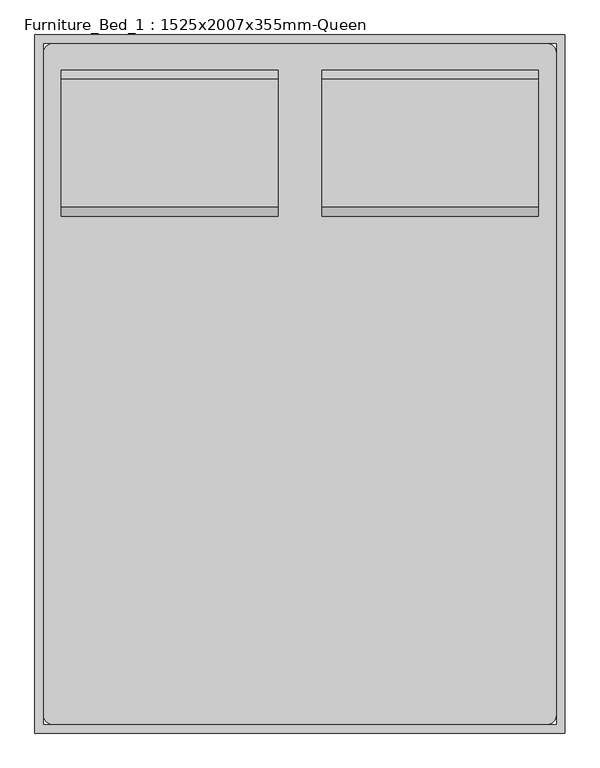
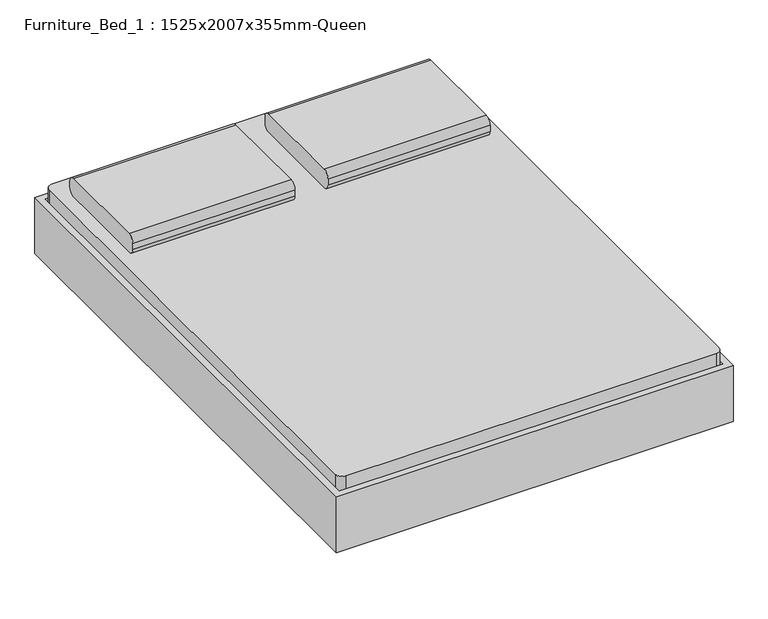
"""IFC4 building model written with IfcOpenShell, lengths in millimetres: furniture geometry, Furniture_Bed_1 : 1525x2007x355mm-Queen."""

from ifc_helpers import new_model, si_unit, point, frame, frame_2d, origin, place, context, project, spatial, polyline, circle_curve, trimmed, segment, composite_curve, outline, extrude, source, transform, mapped, element, save
from ifc_brep_helpers import plane_surface, cylinder_surface, revolved_surface, advanced_brep


def furniture_bed_1_1525x2007x355mm_queen_b7403446(model_context):
    return source(origin(), model_context, "Body", "SolidModel", [
        advanced_brep(
        [(-397.947541, -933.1295082, 196.85), (-397.947541, -933.1295082, 177.8), (-397.947541, -1009.3295082, 177.8), (-397.947541, -1009.3295082, 196.85), (-335.0113525, -933.1295082, 196.85), (-347.147541, -933.1295082, 177.8), (-347.147541, -1009.3295082, 177.8), (-335.0113525, -1009.3295082, 196.85), (-253.8115092, -933.1295082, 22.716374), (-271.0766725, -933.1295082, 14.6654962), (-271.0766725, -1009.3295082, 14.6654962), (-253.8115092, -1009.3295082, 22.716374), (-248.0564547, -933.1295082, 0.0), (-248.0564547, -933.1295082, 19.05), (-248.0564547, -1009.3295082, 0.0), (-248.0564547, -1009.3295082, 19.05), (-169.4439489, -933.1295082, 19.05), (-169.4439489, -933.1295082, 0.0), (-169.4439489, -1009.3295082, 0.0), (-169.4439489, -1009.3295082, 19.05), (-156.7439489, -933.1295082, 3.4029547), (-166.2689489, -933.1295082, 19.9007387), (-156.7439489, -1009.3295082, 3.4029547), (-166.2689489, -1009.3295082, 19.9007387), (-101.7513357, -933.1295082, 57.15), (-96.6469036, -933.1295082, 38.1), (-96.6469036, -1009.3295082, 38.1), (-101.7513357, -1009.3295082, 57.15), (780.0562537, -933.1295082, 57.15), (774.9518216, -933.1295082, 38.1), (774.9518216, -1009.3295082, 38.1), (780.0562537, -1009.3295082, 57.15), (844.5738669, -933.1295082, 19.9007387), (835.0488669, -933.1295082, 3.4029547), (835.0488669, -1009.3295082, 3.4029547), (844.5738669, -1009.3295082, 19.9007387), (847.7488669, -933.1295082, 0.0), (847.7488669, -933.1295082, 19.05), (847.7488669, -1009.3295082, 0.0), (847.7488669, -1009.3295082, 19.05), (926.3613728, -933.1295082, 19.05), (926.3613728, -933.1295082, 0.0), (926.3613728, -1009.3295082, 0.0), (926.3613728, -1009.3295082, 19.05), (949.3815906, -933.1295082, 14.6654962), (932.1164272, -933.1295082, 22.716374), (949.3815906, -1009.3295082, 14.6654962), (932.1164272, -1009.3295082, 22.716374), (1013.3162705, -933.1295082, 196.85), (1025.452459, -933.1295082, 177.8), (1025.452459, -1009.3295082, 177.8), (1013.3162705, -1009.3295082, 196.85), (1076.252459, -933.1295082, 196.85), (1076.252459, -1009.3295082, 196.85), (1076.252459, -1009.3295082, 177.8), (1076.252459, -933.1295082, 177.8)],
        [
            (0, 1),
            (1, 2),
            (2, 3),
            (3, 0),
            (0, 4),
            (4, 5),
            (5, 1),
            (5, 6),
            (6, 2),
            (6, 7),
            (7, 3),
            (7, 4),
            (4, 8),
            (8, 9),
            (9, 5),
            (9, 10),
            (10, 6),
            (10, 11),
            (11, 7),
            (11, 8),
            (12, 9, circle_curve(frame((-248.0564547, -933.1295082, 25.4), z_axis=(0.0, 1.0, 0.0), x_axis=(-0.9063077870366627, 0.0, -0.42261826174067213)), 25.4)),
            (8, 13, circle_curve(frame((-248.0564547, -933.1295082, 25.4), z_axis=(0.0, -1.0, 0.0), x_axis=(-0.9063077870366627, 0.0, -0.42261826174067213)), 6.35)),
            (13, 12),
            (14, 10, circle_curve(frame((-248.0564547, -1009.3295082, 25.4), z_axis=(0.0, 1.0, 0.0), x_axis=(-0.9063077870366627, 0.0, -0.42261826174067213)), 25.4)),
            (12, 14),
            (15, 11, circle_curve(frame((-248.0564547, -1009.3295082, 25.4), z_axis=(0.0, 1.0, 0.0), x_axis=(-0.9063077870366627, 0.0, -0.42261826174067213)), 6.35)),
            (14, 15),
            (15, 13),
            (13, 16),
            (16, 17),
            (17, 12),
            (17, 18),
            (18, 14),
            (18, 19),
            (19, 15),
            (19, 16),
            (20, 17, circle_curve(frame((-169.4439489, -933.1295082, 25.4), z_axis=(0.0, 1.0, 0.0), x_axis=(0.0, 0.0, -1.0)), 25.4)),
            (16, 21, circle_curve(frame((-169.4439489, -933.1295082, 25.4), z_axis=(0.0, -1.0, 0.0), x_axis=(0.0, 0.0, -1.0)), 6.35)),
            (21, 20),
            (22, 18, circle_curve(frame((-169.4439489, -1009.3295082, 25.4), z_axis=(0.0, 1.0, 0.0), x_axis=(0.0, 0.0, -1.0)), 25.4)),
            (20, 22),
            (23, 19, circle_curve(frame((-169.4439489, -1009.3295082, 25.4), z_axis=(0.0, 1.0, 0.0), x_axis=(0.0, 0.0, -1.0)), 6.35)),
            (22, 23),
            (23, 21),
            (21, 24),
            (24, 25),
            (25, 20),
            (25, 26),
            (26, 22),
            (26, 27),
            (27, 23),
            (27, 24),
            (24, 28),
            (28, 29),
            (29, 25),
            (29, 30),
            (30, 26),
            (30, 31),
            (31, 27),
            (31, 28),
            (28, 32),
            (32, 33),
            (33, 29),
            (33, 34),
            (34, 30),
            (34, 35),
            (35, 31),
            (35, 32),
            (36, 33, circle_curve(frame((847.7488669, -933.1295082, 25.4), z_axis=(0.0, 1.0, 0.0), x_axis=(-0.5000000000000486, 0.0, -0.8660254037844105)), 25.4)),
            (32, 37, circle_curve(frame((847.7488669, -933.1295082, 25.4), z_axis=(0.0, -1.0, 0.0), x_axis=(-0.5000000000000486, 0.0, -0.8660254037844105)), 6.35)),
            (37, 36),
            (38, 34, circle_curve(frame((847.7488669, -1009.3295082, 25.4), z_axis=(0.0, 1.0, 0.0), x_axis=(-0.5000000000000486, 0.0, -0.8660254037844105)), 25.4)),
            (36, 38),
            (39, 35, circle_curve(frame((847.7488669, -1009.3295082, 25.4), z_axis=(0.0, 1.0, 0.0), x_axis=(-0.5000000000000486, 0.0, -0.8660254037844105)), 6.35)),
            (38, 39),
            (39, 37),
            (37, 40),
            (40, 41),
            (41, 36),
            (41, 42),
            (42, 38),
            (42, 43),
            (43, 39),
            (43, 40),
            (44, 41, circle_curve(frame((926.3613728, -933.1295082, 25.4), z_axis=(0.0, 1.0, 0.0), x_axis=(0.0, 0.0, -1.0)), 25.4)),
            (40, 45, circle_curve(frame((926.3613728, -933.1295082, 25.4), z_axis=(0.0, -1.0, 0.0), x_axis=(0.0, 0.0, -1.0)), 6.35)),
            (45, 44),
            (46, 42, circle_curve(frame((926.3613728, -1009.3295082, 25.4), z_axis=(0.0, 1.0, 0.0), x_axis=(0.0, 0.0, -1.0)), 25.4)),
            (44, 46),
            (47, 43, circle_curve(frame((926.3613728, -1009.3295082, 25.4), z_axis=(0.0, 1.0, 0.0), x_axis=(0.0, 0.0, -1.0)), 6.35)),
            (46, 47),
            (47, 45),
            (45, 48),
            (48, 49),
            (49, 44),
            (49, 50),
            (50, 46),
            (50, 51),
            (51, 47),
            (51, 48),
            (52, 53),
            (53, 54),
            (54, 55),
            (55, 52),
            (48, 52),
            (55, 49),
            (54, 50),
            (53, 51),
        ],
        [
            plane_surface(frame((-397.947541, -1237.9295082, -127.5947323), z_axis=(-1.0, 0.0, 0.0), x_axis=(0.0, 1.0, 0.0))),
            plane_surface(frame((-397.947541, -933.1295082, 196.85), z_axis=(0.0, 1.0, 0.0), x_axis=(1.0, 0.0, 0.0))),
            plane_surface(frame((-397.947541, -933.1295082, 177.8), z_axis=(0.0, 0.0, -1.0), x_axis=(1.0, 0.0, 0.0))),
            plane_surface(frame((-397.947541, -1009.3295082, 177.8), z_axis=(0.0, -1.0, 0.0), x_axis=(1.0, 0.0, 0.0))),
            plane_surface(frame((-397.947541, -1009.3295082, 196.85), z_axis=(0.0, 0.0, 1.0), x_axis=(1.0, 0.0, 0.0))),
            plane_surface(frame((-335.0113525, -933.1295082, 196.85), z_axis=(0.0, 1.0000000000000002, 0.0), x_axis=(0.4226182617406718, 0.0, -0.9063077870366629))),
            plane_surface(frame((-347.147541, -933.1295082, 177.8), z_axis=(-0.906307787036663, 0.0, -0.4226182617406716), x_axis=(0.4226182617406716, 0.0, -0.906307787036663))),
            plane_surface(frame((-347.147541, -1009.3295082, 177.8), z_axis=(0.0, -1.0000000000000002, 0.0), x_axis=(0.4226182617406718, 0.0, -0.9063077870366629))),
            plane_surface(frame((-335.0113525, -1009.3295082, 196.85), z_axis=(0.9063077870366628, 0.0, 0.42261826174067196), x_axis=(0.42261826174067196, 0.0, -0.9063077870366628))),
            plane_surface(frame((-248.0564547, -933.1295082, 25.4), z_axis=(0.0, 1.0, 0.0), x_axis=(-0.9063077870366627, 0.0, -0.42261826174067213))),
            cylinder_surface(frame((-248.0564547, -1237.9295082, 25.4), z_axis=(0.0, -1.0, 0.0), x_axis=(-0.9063077870366627, 0.0, -0.42261826174067213)), 25.4),
            plane_surface(frame((-248.0564547, -1009.3295082, 25.4), z_axis=(0.0, -1.0, 0.0), x_axis=(-0.9063077870366627, 0.0, -0.42261826174067213))),
            revolved_surface(polyline([(-253.81150914768278, -1009.3295082, 22.716374037946732), (-253.81150914768278, -933.1295082, 22.716374037946732)]), (-248.0564547, -1237.9295082, 25.4), (0.0, -1.0, 0.0)),
            plane_surface(frame((-248.0564547, -933.1295082, 19.05), z_axis=(0.0, 1.0, 0.0), x_axis=(1.0, 0.0, 0.0))),
            plane_surface(frame((-248.0564547, -933.1295082, 0.0), z_axis=(0.0, 0.0, -1.0), x_axis=(1.0, 0.0, 0.0))),
            plane_surface(frame((-248.0564547, -1009.3295082, 0.0), z_axis=(0.0, -1.0, 0.0), x_axis=(1.0, 0.0, 0.0))),
            plane_surface(frame((-248.0564547, -1009.3295082, 19.05), z_axis=(0.0, 0.0, 1.0), x_axis=(1.0, 0.0, 0.0))),
            plane_surface(frame((-169.4439489, -933.1295082, 25.4), z_axis=(0.0, 1.0, 0.0), x_axis=(0.0, 0.0, -1.0))),
            cylinder_surface(frame((-169.4439489, -1237.9295082, 25.4), z_axis=(0.0, -1.0, 0.0), x_axis=(0.0, 0.0, -1.0)), 25.4),
            plane_surface(frame((-169.4439489, -1009.3295082, 25.4), z_axis=(0.0, -1.0, 0.0), x_axis=(0.0, 0.0, -1.0))),
            revolved_surface(polyline([(-169.4439489, -1009.3295082, 19.049999999999997), (-169.4439489, -933.1295082, 19.049999999999997)]), (-169.4439489, -1237.9295082, 25.4), (0.0, -1.0, 0.0)),
            plane_surface(frame((-166.2689489, -933.1295082, 19.9007387), z_axis=(0.0, 1.0, 0.0), x_axis=(0.8660254037844786, 0.0, 0.4999999999999309))),
            plane_surface(frame((-156.7439489, -933.1295082, 3.4029547), z_axis=(0.4999999999999315, 0.0, -0.8660254037844782), x_axis=(0.8660254037844782, 0.0, 0.4999999999999315))),
            plane_surface(frame((-156.7439489, -1009.3295082, 3.4029547), z_axis=(0.0, -1.0, 0.0), x_axis=(0.8660254037844788, 0.0, 0.49999999999993044))),
            plane_surface(frame((-166.2689489, -1009.3295082, 19.9007387), z_axis=(-0.4999999999999304, 0.0, 0.8660254037844789), x_axis=(0.8660254037844789, 0.0, 0.4999999999999304))),
            plane_surface(frame((-101.7513357, -933.1295082, 57.15), z_axis=(0.0, 1.0, 0.0), x_axis=(1.0, 0.0, 0.0))),
            plane_surface(frame((-96.6469036, -933.1295082, 38.1), z_axis=(0.0, 0.0, -1.0), x_axis=(1.0, 0.0, 0.0))),
            plane_surface(frame((-96.6469036, -1009.3295082, 38.1), z_axis=(0.0, -1.0, 0.0), x_axis=(1.0, 0.0, 0.0))),
            plane_surface(frame((-101.7513357, -1009.3295082, 57.15), z_axis=(0.0, 0.0, 1.0), x_axis=(1.0, 0.0, 0.0))),
            plane_surface(frame((780.0562537, -933.1295082, 57.15), z_axis=(0.0, 1.0, 0.0), x_axis=(0.866025403784412, 0.0, -0.5000000000000463))),
            plane_surface(frame((774.9518216, -933.1295082, 38.1), z_axis=(-0.500000000000047, 0.0, -0.8660254037844116), x_axis=(0.8660254037844116, 0.0, -0.500000000000047))),
            plane_surface(frame((774.9518216, -1009.3295082, 38.1), z_axis=(0.0, -1.0, 0.0), x_axis=(0.866025403784411, 0.0, -0.5000000000000481))),
            plane_surface(frame((780.0562537, -1009.3295082, 57.15), z_axis=(0.5000000000000471, 0.0, 0.8660254037844115), x_axis=(0.8660254037844115, 0.0, -0.5000000000000471))),
            plane_surface(frame((847.7488669, -933.1295082, 25.4), z_axis=(0.0, 1.0000000000000002, 0.0), x_axis=(-0.5000000000000487, 0.0, -0.8660254037844106))),
            cylinder_surface(frame((847.7488669, -1237.9295082, 25.4), z_axis=(0.0, -1.0, 0.0), x_axis=(-0.5000000000000486, 0.0, -0.8660254037844105)), 25.4),
            plane_surface(frame((847.7488669, -1009.3295082, 25.4), z_axis=(0.0, -1.0000000000000002, 0.0), x_axis=(-0.5000000000000487, 0.0, -0.8660254037844106))),
            revolved_surface(polyline([(844.5738668999998, -1009.3295082, 19.900738685968992), (844.5738668999998, -933.1295082, 19.900738685968992)]), (847.7488669, -1237.9295082, 25.4), (0.0, -1.0, 0.0)),
            plane_surface(frame((847.7488669, -933.1295082, 19.05), z_axis=(0.0, 1.0, 0.0), x_axis=(1.0, 0.0, 0.0))),
            plane_surface(frame((847.7488669, -933.1295082, 0.0), z_axis=(0.0, 0.0, -1.0), x_axis=(1.0, 0.0, 0.0))),
            plane_surface(frame((847.7488669, -1009.3295082, 0.0), z_axis=(0.0, -1.0, 0.0), x_axis=(1.0, 0.0, 0.0))),
            plane_surface(frame((847.7488669, -1009.3295082, 19.05), z_axis=(0.0, 0.0, 1.0), x_axis=(1.0, 0.0, 0.0))),
            plane_surface(frame((926.3613728, -933.1295082, 25.4), z_axis=(0.0, 1.0, 0.0), x_axis=(0.0, 0.0, -1.0))),
            cylinder_surface(frame((926.3613728, -1237.9295082, 25.4), z_axis=(0.0, -1.0, 0.0), x_axis=(0.0, 0.0, -1.0)), 25.4),
            plane_surface(frame((926.3613728, -1009.3295082, 25.4), z_axis=(0.0, -1.0, 0.0), x_axis=(0.0, 0.0, -1.0))),
            revolved_surface(polyline([(926.3613728, -1009.3295082, 19.049999999999997), (926.3613728, -933.1295082, 19.049999999999997)]), (926.3613728, -1237.9295082, 25.4), (0.0, -1.0, 0.0)),
            plane_surface(frame((932.1164272, -933.1295082, 22.716374), z_axis=(0.0, 1.0, 0.0), x_axis=(0.4226182617405395, 0.0, 0.9063077870367245))),
            plane_surface(frame((949.3815906, -933.1295082, 14.6654962), z_axis=(0.9063077870367247, 0.0, -0.4226182617405394), x_axis=(0.4226182617405394, 0.0, 0.9063077870367247))),
            plane_surface(frame((949.3815906, -1009.3295082, 14.6654962), z_axis=(0.0, -1.0, 0.0), x_axis=(0.4226182617405393, 0.0, 0.9063077870367247))),
            plane_surface(frame((932.1164272, -1009.3295082, 22.716374), z_axis=(-0.9063077870367245, 0.0, 0.42261826174053974), x_axis=(0.42261826174053974, 0.0, 0.9063077870367245))),
            plane_surface(frame((1076.252459, -1237.9295082, -127.5947323), z_axis=(1.0, 0.0, 0.0), x_axis=(0.0, 1.0, 0.0))),
            plane_surface(frame((1013.3162705, -933.1295082, 196.85), z_axis=(0.0, 1.0, 0.0), x_axis=(1.0, 0.0, 0.0))),
            plane_surface(frame((1025.452459, -933.1295082, 177.8), z_axis=(0.0, 0.0, -1.0), x_axis=(1.0, 0.0, 0.0))),
            plane_surface(frame((1025.452459, -1009.3295082, 177.8), z_axis=(0.0, -1.0, 0.0), x_axis=(1.0, 0.0, 0.0))),
            plane_surface(frame((1013.3162705, -1009.3295082, 196.85), z_axis=(0.0, 0.0, 1.0), x_axis=(1.0, 0.0, 0.0))),
        ],
        [
            (0, [[1, 2, 3, 4]]),
            (1, [[-1, 5, 6, 7]]),
            (2, [[-2, -7, 8, 9]]),
            (3, [[-3, -9, 10, 11]]),
            (4, [[-4, -11, 12, -5]]),
            (5, [[-6, 13, 14, 15]]),
            (6, [[-8, -15, 16, 17]]),
            (7, [[-10, -17, 18, 19]]),
            (8, [[-12, -19, 20, -13]]),
            (9, [[21, -14, 22, 23]]),
            (10, [[24, -16, -21, 25]]),
            (11, [[26, -18, -24, 27]]),
            (12, [[-22, -20, -26, 28]]),
            (13, [[-23, 29, 30, 31]]),
            (14, [[-25, -31, 32, 33]]),
            (15, [[-27, -33, 34, 35]]),
            (16, [[-28, -35, 36, -29]]),
            (17, [[37, -30, 38, 39]]),
            (18, [[40, -32, -37, 41]]),
            (19, [[42, -34, -40, 43]]),
            (20, [[-38, -36, -42, 44]]),
            (21, [[-39, 45, 46, 47]]),
            (22, [[-41, -47, 48, 49]]),
            (23, [[-43, -49, 50, 51]]),
            (24, [[-44, -51, 52, -45]]),
            (25, [[-46, 53, 54, 55]]),
            (26, [[-48, -55, 56, 57]]),
            (27, [[-50, -57, 58, 59]]),
            (28, [[-52, -59, 60, -53]]),
            (29, [[-54, 61, 62, 63]]),
            (30, [[-56, -63, 64, 65]]),
            (31, [[-58, -65, 66, 67]]),
            (32, [[-60, -67, 68, -61]]),
            (33, [[69, -62, 70, 71]]),
            (34, [[72, -64, -69, 73]]),
            (35, [[74, -66, -72, 75]]),
            (36, [[-70, -68, -74, 76]]),
            (37, [[-71, 77, 78, 79]]),
            (38, [[-73, -79, 80, 81]]),
            (39, [[-75, -81, 82, 83]]),
            (40, [[-76, -83, 84, -77]]),
            (41, [[85, -78, 86, 87]]),
            (42, [[88, -80, -85, 89]]),
            (43, [[90, -82, -88, 91]]),
            (44, [[-86, -84, -90, 92]]),
            (45, [[-87, 93, 94, 95]]),
            (46, [[-89, -95, 96, 97]]),
            (47, [[-91, -97, 98, 99]]),
            (48, [[-92, -99, 100, -93]]),
            (49, [[101, 102, 103, 104]]),
            (50, [[-94, 105, -104, 106]]),
            (51, [[-96, -106, -103, 107]]),
            (52, [[-98, -107, -102, 108]]),
            (53, [[-100, -108, -101, -105]]),
        ],
    ),
        extrude(outline(composite_curve([segment(polyline([(-372.547541, 743.6704918), (1050.852459, 743.6704918)]), True, "CONTINUOUS"), segment(trimmed(circle_curve(frame_2d((1050.852459, 718.2704918)), 25.4), [point((1050.852459, 743.6704918))], [point((1076.252459, 718.2704918))], False, "CARTESIAN"), True, "CONTINUOUS"), segment(polyline([(1076.252459, 718.2704918), (1076.252459, -1187.1295082)]), True, "CONTINUOUS"), segment(trimmed(circle_curve(frame_2d((1050.852459, -1187.1295082)), 25.4), [point((1076.252459, -1187.1295082))], [point((1050.852459, -1212.5295082))], False, "CARTESIAN"), True, "CONTINUOUS"), segment(polyline([(1050.852459, -1212.5295082), (-372.547541, -1212.5295082)]), True, "CONTINUOUS"), segment(trimmed(circle_curve(frame_2d((-372.547541, -1187.1295082)), 25.4), [point((-372.547541, -1212.5295082))], [point((-397.947541, -1187.1295082))], False, "CARTESIAN"), True, "CONTINUOUS"), segment(polyline([(-397.947541, -1187.1295082), (-397.947541, 718.2704918)]), True, "CONTINUOUS"), segment(trimmed(circle_curve(frame_2d((-372.547541, 718.2704918)), 25.4), [point((-397.947541, 718.2704918))], [point((-372.547541, 743.6704918))], False, "CARTESIAN"), True, "CONTINUOUS")], self_intersect=False)), frame((0.0, 0.0, 203.2), z_axis=(0.0, 0.0, 1.0), x_axis=(1.0, 0.0, 0.0)), (0.0, 0.0, 1.0), 203.2),
        advanced_brep(
        [(-397.6231784, 515.0704918, 177.8), (-397.6231784, 438.8704918, 177.8), (-397.6231784, 438.8704918, 196.85), (-397.6231784, 515.0704918, 196.85), (-346.8231784, 515.0704918, 177.8), (-346.8231784, 438.8704918, 177.8), (-334.6869899, 438.8704918, 196.85), (-334.6869899, 515.0704918, 196.85), (-270.7523099, 515.0704918, 14.6654962), (-270.7523099, 438.8704918, 14.6654962), (-253.4871466, 438.8704918, 22.716374), (-253.4871466, 515.0704918, 22.716374), (-247.7320921, 438.8704918, 0.0), (-247.7320921, 515.0704918, 0.0), (-247.7320921, 438.8704918, 19.05), (-247.7320921, 515.0704918, 19.05), (-169.1195862, 515.0704918, 0.0), (-169.1195862, 438.8704918, 0.0), (-169.1195862, 438.8704918, 19.05), (-169.1195862, 515.0704918, 19.05), (-156.4195862, 438.8704918, 3.4029547), (-156.4195862, 515.0704918, 3.4029547), (-165.9445862, 438.8704918, 19.9007387), (-165.9445862, 515.0704918, 19.9007387), (-96.322541, 515.0704918, 38.1), (-96.322541, 438.8704918, 38.1), (-101.4269731, 438.8704918, 57.15), (-101.4269731, 515.0704918, 57.15), (774.9518216, 515.0704918, 38.1), (774.9518216, 438.8704918, 38.1), (780.0562537, 438.8704918, 57.15), (780.0562537, 515.0704918, 57.15), (835.0488669, 515.0704918, 3.4029547), (835.0488669, 438.8704918, 3.4029547), (844.5738669, 438.8704918, 19.9007387), (844.5738669, 515.0704918, 19.9007387), (847.7488669, 438.8704918, 0.0), (847.7488669, 515.0704918, 0.0), (847.7488669, 438.8704918, 19.05), (847.7488669, 515.0704918, 19.05), (926.3613728, 515.0704918, 0.0), (926.3613728, 438.8704918, 0.0), (926.3613728, 438.8704918, 19.05), (926.3613728, 515.0704918, 19.05), (949.3815906, 438.8704918, 14.6654962), (949.3815906, 515.0704918, 14.6654962), (932.1164272, 438.8704918, 22.716374), (932.1164272, 515.0704918, 22.716374), (1025.452459, 515.0704918, 177.8), (1025.452459, 438.8704918, 177.8), (1013.3162705, 438.8704918, 196.85), (1013.3162705, 515.0704918, 196.85), (1076.252459, 515.0704918, 177.8), (1076.252459, 515.0704918, 196.85), (1076.252459, 438.8704918, 196.85), (1076.252459, 438.8704918, 177.8)],
        [
            (0, 1),
            (1, 2),
            (2, 3),
            (3, 0),
            (0, 4),
            (4, 5),
            (5, 1),
            (5, 6),
            (6, 2),
            (6, 7),
            (7, 3),
            (7, 4),
            (4, 8),
            (8, 9),
            (9, 5),
            (9, 10),
            (10, 6),
            (10, 11),
            (11, 7),
            (11, 8),
            (12, 9, circle_curve(frame((-247.7320921, 438.8704918, 25.4), z_axis=(0.0, 1.0, 0.0), x_axis=(-0.906307787036649, 0.0, -0.4226182617407015)), 25.4)),
            (8, 13, circle_curve(frame((-247.7320921, 515.0704918, 25.4), z_axis=(0.0, -1.0, 0.0), x_axis=(-0.906307787036649, 0.0, -0.4226182617407015)), 25.4)),
            (13, 12),
            (14, 10, circle_curve(frame((-247.7320921, 438.8704918, 25.4), z_axis=(0.0, 1.0, 0.0), x_axis=(-0.906307787036649, 0.0, -0.4226182617407015)), 6.35)),
            (12, 14),
            (15, 11, circle_curve(frame((-247.7320921, 515.0704918, 25.4), z_axis=(0.0, 1.0, 0.0), x_axis=(-0.906307787036649, 0.0, -0.4226182617407015)), 6.35)),
            (14, 15),
            (15, 13),
            (13, 16),
            (16, 17),
            (17, 12),
            (17, 18),
            (18, 14),
            (18, 19),
            (19, 15),
            (19, 16),
            (20, 17, circle_curve(frame((-169.1195862, 438.8704918, 25.4), z_axis=(0.0, 1.0, 0.0), x_axis=(0.0, 0.0, -1.0)), 25.4)),
            (16, 21, circle_curve(frame((-169.1195862, 515.0704918, 25.4), z_axis=(0.0, -1.0, 0.0), x_axis=(0.0, 0.0, -1.0)), 25.4)),
            (21, 20),
            (22, 18, circle_curve(frame((-169.1195862, 438.8704918, 25.4), z_axis=(0.0, 1.0, 0.0), x_axis=(0.0, 0.0, -1.0)), 6.35)),
            (20, 22),
            (23, 19, circle_curve(frame((-169.1195862, 515.0704918, 25.4), z_axis=(0.0, 1.0, 0.0), x_axis=(0.0, 0.0, -1.0)), 6.35)),
            (22, 23),
            (23, 21),
            (21, 24),
            (24, 25),
            (25, 20),
            (25, 26),
            (26, 22),
            (26, 27),
            (27, 23),
            (27, 24),
            (24, 28),
            (28, 29),
            (29, 25),
            (29, 30),
            (30, 26),
            (30, 31),
            (31, 27),
            (31, 28),
            (28, 32),
            (32, 33),
            (33, 29),
            (33, 34),
            (34, 30),
            (34, 35),
            (35, 31),
            (35, 32),
            (36, 33, circle_curve(frame((847.7488669, 438.8704918, 25.4), z_axis=(0.0, 1.0, 0.0), x_axis=(-0.5000000000000444, 0.0, -0.866025403784413)), 25.4)),
            (32, 37, circle_curve(frame((847.7488669, 515.0704918, 25.4), z_axis=(0.0, -1.0, 0.0), x_axis=(-0.5000000000000444, 0.0, -0.866025403784413)), 25.4)),
            (37, 36),
            (38, 34, circle_curve(frame((847.7488669, 438.8704918, 25.4), z_axis=(0.0, 1.0, 0.0), x_axis=(-0.5000000000000444, 0.0, -0.866025403784413)), 6.35)),
            (36, 38),
            (39, 35, circle_curve(frame((847.7488669, 515.0704918, 25.4), z_axis=(0.0, 1.0, 0.0), x_axis=(-0.5000000000000444, 0.0, -0.866025403784413)), 6.35)),
            (38, 39),
            (39, 37),
            (37, 40),
            (40, 41),
            (41, 36),
            (41, 42),
            (42, 38),
            (42, 43),
            (43, 39),
            (43, 40),
            (44, 41, circle_curve(frame((926.3613728, 438.8704918, 25.4), z_axis=(0.0, 1.0, 0.0), x_axis=(0.0, 0.0, -1.0)), 25.4)),
            (40, 45, circle_curve(frame((926.3613728, 515.0704918, 25.4), z_axis=(0.0, -1.0, 0.0), x_axis=(0.0, 0.0, -1.0)), 25.4)),
            (45, 44),
            (46, 42, circle_curve(frame((926.3613728, 438.8704918, 25.4), z_axis=(0.0, 1.0, 0.0), x_axis=(0.0, 0.0, -1.0)), 6.35)),
            (44, 46),
            (47, 43, circle_curve(frame((926.3613728, 515.0704918, 25.4), z_axis=(0.0, 1.0, 0.0), x_axis=(0.0, 0.0, -1.0)), 6.35)),
            (46, 47),
            (47, 45),
            (45, 48),
            (48, 49),
            (49, 44),
            (49, 50),
            (50, 46),
            (50, 51),
            (51, 47),
            (51, 48),
            (52, 53),
            (53, 54),
            (54, 55),
            (55, 52),
            (48, 52),
            (55, 49),
            (54, 50),
            (53, 51),
        ],
        [
            plane_surface(frame((-397.6231784, 769.0704918, -152.9490627), z_axis=(-1.0, 0.0, 0.0), x_axis=(0.0, 1.0, 0.0))),
            plane_surface(frame((-397.6231784, 515.0704918, 177.8), z_axis=(0.0, 0.0, -1.0), x_axis=(1.0, 0.0, 0.0))),
            plane_surface(frame((-397.6231784, 438.8704918, 177.8), z_axis=(0.0, -1.0, 0.0), x_axis=(1.0, 0.0, 0.0))),
            plane_surface(frame((-397.6231784, 438.8704918, 196.85), z_axis=(0.0, 0.0, 1.0), x_axis=(1.0, 0.0, 0.0))),
            plane_surface(frame((-397.6231784, 515.0704918, 196.85), z_axis=(0.0, 1.0, 0.0), x_axis=(1.0, 0.0, 0.0))),
            plane_surface(frame((-346.8231784, 515.0704918, 177.8), z_axis=(-0.9063077870366485, 0.0, -0.4226182617407029), x_axis=(0.4226182617407029, 0.0, -0.9063077870366485))),
            plane_surface(frame((-346.8231784, 438.8704918, 177.8), z_axis=(0.0, -1.0, 0.0), x_axis=(0.42261826174070266, 0.0, -0.9063077870366485))),
            plane_surface(frame((-334.6869899, 438.8704918, 196.85), z_axis=(0.9063077870366486, 0.0, 0.4226182617407026), x_axis=(0.4226182617407026, 0.0, -0.9063077870366486))),
            plane_surface(frame((-334.6869899, 515.0704918, 196.85), z_axis=(0.0, 1.0, 0.0), x_axis=(0.42261826174070266, 0.0, -0.9063077870366485))),
            cylinder_surface(frame((-247.7320921, 769.0704918, 25.4), z_axis=(0.0, -1.0, 0.0), x_axis=(-0.906307787036649, 0.0, -0.4226182617407015)), 25.4),
            plane_surface(frame((-247.7320921, 438.8704918, 25.4), z_axis=(0.0, -1.0, 0.0), x_axis=(-0.906307787036649, 0.0, -0.4226182617407015))),
            revolved_surface(polyline([(-253.4871465476827, 438.8704918, 22.716374037946544), (-253.4871465476827, 515.0704918, 22.716374037946544)]), (-247.7320921, 769.0704918, 25.4), (0.0, -1.0, 0.0)),
            plane_surface(frame((-247.7320921, 515.0704918, 25.4), z_axis=(0.0, 1.0, 0.0), x_axis=(-0.906307787036649, 0.0, -0.4226182617407015))),
            plane_surface(frame((-247.7320921, 515.0704918, 0.0), z_axis=(0.0, 0.0, -1.0), x_axis=(1.0, 0.0, 0.0))),
            plane_surface(frame((-247.7320921, 438.8704918, 0.0), z_axis=(0.0, -1.0, 0.0), x_axis=(1.0, 0.0, 0.0))),
            plane_surface(frame((-247.7320921, 438.8704918, 19.05), z_axis=(0.0, 0.0, 1.0), x_axis=(1.0, 0.0, 0.0))),
            plane_surface(frame((-247.7320921, 515.0704918, 19.05), z_axis=(0.0, 1.0, 0.0), x_axis=(1.0, 0.0, 0.0))),
            cylinder_surface(frame((-169.1195862, 769.0704918, 25.4), z_axis=(0.0, -1.0, 0.0), x_axis=(0.0, 0.0, -1.0)), 25.4),
            plane_surface(frame((-169.1195862, 438.8704918, 25.4), z_axis=(0.0, -1.0, 0.0), x_axis=(0.0, 0.0, -1.0))),
            revolved_surface(polyline([(-169.1195862, 438.8704918, 19.049999999999997), (-169.1195862, 515.0704918, 19.049999999999997)]), (-169.1195862, 769.0704918, 25.4), (0.0, -1.0, 0.0)),
            plane_surface(frame((-169.1195862, 515.0704918, 25.4), z_axis=(0.0, 1.0, 0.0), x_axis=(0.0, 0.0, -1.0))),
            plane_surface(frame((-156.4195862, 515.0704918, 3.4029547), z_axis=(0.49999999999987826, 0.0, -0.866025403784509), x_axis=(0.866025403784509, 0.0, 0.49999999999987826))),
            plane_surface(frame((-156.4195862, 438.8704918, 3.4029547), z_axis=(0.0, -1.0, 0.0), x_axis=(0.8660254037845093, 0.0, 0.4999999999998776))),
            plane_surface(frame((-165.9445862, 438.8704918, 19.9007387), z_axis=(-0.4999999999998785, 0.0, 0.8660254037845089), x_axis=(0.8660254037845089, 0.0, 0.4999999999998785))),
            plane_surface(frame((-165.9445862, 515.0704918, 19.9007387), z_axis=(0.0, 1.0, 0.0), x_axis=(0.866025403784509, 0.0, 0.49999999999987826))),
            plane_surface(frame((-96.322541, 515.0704918, 38.1), z_axis=(0.0, 0.0, -1.0), x_axis=(1.0, 0.0, 0.0))),
            plane_surface(frame((-96.322541, 438.8704918, 38.1), z_axis=(0.0, -1.0, 0.0), x_axis=(1.0, 0.0, 0.0))),
            plane_surface(frame((-101.4269731, 438.8704918, 57.15), z_axis=(0.0, 0.0, 1.0), x_axis=(1.0, 0.0, 0.0))),
            plane_surface(frame((-101.4269731, 515.0704918, 57.15), z_axis=(0.0, 1.0, 0.0), x_axis=(1.0, 0.0, 0.0))),
            plane_surface(frame((774.9518216, 515.0704918, 38.1), z_axis=(-0.5000000000000451, 0.0, -0.8660254037844127), x_axis=(0.8660254037844127, 0.0, -0.5000000000000451))),
            plane_surface(frame((774.9518216, 438.8704918, 38.1), z_axis=(0.0, -1.0, 0.0), x_axis=(0.866025403784413, 0.0, -0.5000000000000446))),
            plane_surface(frame((780.0562537, 438.8704918, 57.15), z_axis=(0.5000000000000449, 0.0, 0.8660254037844127), x_axis=(0.8660254037844127, 0.0, -0.5000000000000449))),
            plane_surface(frame((780.0562537, 515.0704918, 57.15), z_axis=(0.0, 1.0, 0.0), x_axis=(0.8660254037844125, 0.0, -0.5000000000000454))),
            cylinder_surface(frame((847.7488669, 769.0704918, 25.4), z_axis=(0.0, -1.0, 0.0), x_axis=(-0.5000000000000444, 0.0, -0.866025403784413)), 25.4),
            plane_surface(frame((847.7488669, 438.8704918, 25.4), z_axis=(0.0, -1.0000000000000002, 0.0), x_axis=(-0.5000000000000445, 0.0, -0.8660254037844131))),
            revolved_surface(polyline([(844.5738668999998, 438.8704918, 19.900738685968975), (844.5738668999998, 515.0704918, 19.900738685968975)]), (847.7488669, 769.0704918, 25.4), (0.0, -1.0, 0.0)),
            plane_surface(frame((847.7488669, 515.0704918, 25.4), z_axis=(0.0, 1.0000000000000002, 0.0), x_axis=(-0.5000000000000445, 0.0, -0.8660254037844131))),
            plane_surface(frame((847.7488669, 515.0704918, 0.0), z_axis=(0.0, 0.0, -1.0), x_axis=(1.0, 0.0, 0.0))),
            plane_surface(frame((847.7488669, 438.8704918, 0.0), z_axis=(0.0, -1.0, 0.0), x_axis=(1.0, 0.0, 0.0))),
            plane_surface(frame((847.7488669, 438.8704918, 19.05), z_axis=(0.0, 0.0, 1.0), x_axis=(1.0, 0.0, 0.0))),
            plane_surface(frame((847.7488669, 515.0704918, 19.05), z_axis=(0.0, 1.0, 0.0), x_axis=(1.0, 0.0, 0.0))),
            cylinder_surface(frame((926.3613728, 769.0704918, 25.4), z_axis=(0.0, -1.0, 0.0), x_axis=(0.0, 0.0, -1.0)), 25.4),
            plane_surface(frame((926.3613728, 438.8704918, 25.4), z_axis=(0.0, -1.0, 0.0), x_axis=(0.0, 0.0, -1.0))),
            revolved_surface(polyline([(926.3613728, 438.8704918, 19.049999999999997), (926.3613728, 515.0704918, 19.049999999999997)]), (926.3613728, 769.0704918, 25.4), (0.0, -1.0, 0.0)),
            plane_surface(frame((926.3613728, 515.0704918, 25.4), z_axis=(0.0, 1.0, 0.0), x_axis=(0.0, 0.0, -1.0))),
            plane_surface(frame((949.3815906, 515.0704918, 14.6654962), z_axis=(0.9063077870366802, 0.0, -0.4226182617406346), x_axis=(0.4226182617406346, 0.0, 0.9063077870366802))),
            plane_surface(frame((949.3815906, 438.8704918, 14.6654962), z_axis=(0.0, -1.0, 0.0), x_axis=(0.42261826174063377, 0.0, 0.9063077870366806))),
            plane_surface(frame((932.1164272, 438.8704918, 22.716374), z_axis=(-0.9063077870366807, 0.0, 0.4226182617406337), x_axis=(0.4226182617406337, 0.0, 0.9063077870366807))),
            plane_surface(frame((932.1164272, 515.0704918, 22.716374), z_axis=(0.0, 1.0, 0.0), x_axis=(0.4226182617406339, 0.0, 0.9063077870366806))),
            plane_surface(frame((1076.252459, 769.0704918, -152.9490627), z_axis=(1.0, 0.0, 0.0), x_axis=(0.0, 1.0, 0.0))),
            plane_surface(frame((1025.452459, 515.0704918, 177.8), z_axis=(0.0, 0.0, -1.0), x_axis=(1.0, 0.0, 0.0))),
            plane_surface(frame((1025.452459, 438.8704918, 177.8), z_axis=(0.0, -1.0, 0.0), x_axis=(1.0, 0.0, 0.0))),
            plane_surface(frame((1013.3162705, 438.8704918, 196.85), z_axis=(0.0, 0.0, 1.0), x_axis=(1.0, 0.0, 0.0))),
            plane_surface(frame((1013.3162705, 515.0704918, 196.85), z_axis=(0.0, 1.0, 0.0), x_axis=(1.0, 0.0, 0.0))),
        ],
        [
            (0, [[1, 2, 3, 4]]),
            (1, [[-1, 5, 6, 7]]),
            (2, [[-2, -7, 8, 9]]),
            (3, [[-3, -9, 10, 11]]),
            (4, [[-4, -11, 12, -5]]),
            (5, [[-6, 13, 14, 15]]),
            (6, [[-8, -15, 16, 17]]),
            (7, [[-10, -17, 18, 19]]),
            (8, [[-12, -19, 20, -13]]),
            (9, [[21, -14, 22, 23]]),
            (10, [[24, -16, -21, 25]]),
            (11, [[26, -18, -24, 27]]),
            (12, [[-22, -20, -26, 28]]),
            (13, [[-23, 29, 30, 31]]),
            (14, [[-25, -31, 32, 33]]),
            (15, [[-27, -33, 34, 35]]),
            (16, [[-28, -35, 36, -29]]),
            (17, [[37, -30, 38, 39]]),
            (18, [[40, -32, -37, 41]]),
            (19, [[42, -34, -40, 43]]),
            (20, [[-38, -36, -42, 44]]),
            (21, [[-39, 45, 46, 47]]),
            (22, [[-41, -47, 48, 49]]),
            (23, [[-43, -49, 50, 51]]),
            (24, [[-44, -51, 52, -45]]),
            (25, [[-46, 53, 54, 55]]),
            (26, [[-48, -55, 56, 57]]),
            (27, [[-50, -57, 58, 59]]),
            (28, [[-52, -59, 60, -53]]),
            (29, [[-54, 61, 62, 63]]),
            (30, [[-56, -63, 64, 65]]),
            (31, [[-58, -65, 66, 67]]),
            (32, [[-60, -67, 68, -61]]),
            (33, [[69, -62, 70, 71]]),
            (34, [[72, -64, -69, 73]]),
            (35, [[74, -66, -72, 75]]),
            (36, [[-70, -68, -74, 76]]),
            (37, [[-71, 77, 78, 79]]),
            (38, [[-73, -79, 80, 81]]),
            (39, [[-75, -81, 82, 83]]),
            (40, [[-76, -83, 84, -77]]),
            (41, [[85, -78, 86, 87]]),
            (42, [[88, -80, -85, 89]]),
            (43, [[90, -82, -88, 91]]),
            (44, [[-86, -84, -90, 92]]),
            (45, [[-87, 93, 94, 95]]),
            (46, [[-89, -95, 96, 97]]),
            (47, [[-91, -97, 98, 99]]),
            (48, [[-92, -99, 100, -93]]),
            (49, [[101, 102, 103, 104]]),
            (50, [[-94, 105, -104, 106]]),
            (51, [[-96, -106, -103, 107]]),
            (52, [[-98, -107, -102, 108]]),
            (53, [[-100, -108, -101, -105]]),
        ],
    ),
        extrude(outline(composite_curve([segment(polyline([(642.0704918, 406.4), (273.7704918, 406.4)]), True, "CONTINUOUS"), segment(trimmed(circle_curve(frame_2d((273.7704918, 431.8)), 25.4), [point((273.7704918, 406.4))], [point((248.3704918, 431.8))], False, "CARTESIAN"), True, "CONTINUOUS"), segment(polyline([(248.3704918, 431.8), (248.3704918, 457.2)]), True, "CONTINUOUS"), segment(trimmed(circle_curve(frame_2d((273.7704918, 457.2)), 25.4), [point((248.3704918, 457.2))], [point((273.7704918, 482.6))], False, "CARTESIAN"), True, "CONTINUOUS"), segment(polyline([(273.7704918, 482.6), (642.0704918, 482.6)]), True, "CONTINUOUS"), segment(trimmed(circle_curve(frame_2d((642.0704918, 457.2)), 25.4), [point((642.0704918, 482.6))], [point((667.4704918, 457.2))], False, "CARTESIAN"), True, "CONTINUOUS"), segment(polyline([(667.4704918, 457.2), (667.4704918, 431.8)]), True, "CONTINUOUS"), segment(trimmed(circle_curve(frame_2d((642.0704918, 431.8)), 25.4), [point((667.4704918, 431.8))], [point((642.0704918, 406.4))], False, "CARTESIAN"), True, "CONTINUOUS")], self_intersect=False)), frame((-347.147541, 0.0, 0.0), z_axis=(1.0, 0.0, 0.0), x_axis=(0.0, 1.0, 0.0)), (0.0, 0.0, 1.0), 622.8),
        extrude(outline(composite_curve([segment(polyline([(642.0704918, 406.4), (273.7704918, 406.4)]), True, "CONTINUOUS"), segment(trimmed(circle_curve(frame_2d((273.7704918, 431.8)), 25.4), [point((273.7704918, 406.4))], [point((248.3704918, 431.8))], False, "CARTESIAN"), True, "CONTINUOUS"), segment(polyline([(248.3704918, 431.8), (248.3704918, 457.2)]), True, "CONTINUOUS"), segment(trimmed(circle_curve(frame_2d((273.7704918, 457.2)), 25.4), [point((248.3704918, 457.2))], [point((273.7704918, 482.6))], False, "CARTESIAN"), True, "CONTINUOUS"), segment(polyline([(273.7704918, 482.6), (642.0704918, 482.6)]), True, "CONTINUOUS"), segment(trimmed(circle_curve(frame_2d((642.0704918, 457.2)), 25.4), [point((642.0704918, 482.6))], [point((667.4704918, 457.2))], False, "CARTESIAN"), True, "CONTINUOUS"), segment(polyline([(667.4704918, 457.2), (667.4704918, 431.8)]), True, "CONTINUOUS"), segment(trimmed(circle_curve(frame_2d((642.0704918, 431.8)), 25.4), [point((667.4704918, 431.8))], [point((642.0704918, 406.4))], False, "CARTESIAN"), True, "CONTINUOUS")], self_intersect=False)), frame((402.652459, 0.0, 0.0), z_axis=(1.0, 0.0, 0.0), x_axis=(0.0, 1.0, 0.0)), (0.0, 0.0, 1.0), 622.8),
        extrude(outline(polyline([(1101.652459, 769.0704918), (1101.652459, -1237.9295082), (-423.347541, -1237.9295082), (-423.347541, 769.0704918), (1101.652459, 769.0704918)]), holes=[polyline([(1076.252459, 743.6704918), (-397.947541, 743.6704918), (-397.947541, -1212.5295082), (1076.252459, -1212.5295082), (1076.252459, 743.6704918)])]), frame((0.0, 0.0, 127.0), z_axis=(0.0, 0.0, 1.0), x_axis=(1.0, 0.0, 0.0)), (0.0, 0.0, 1.0), 228.6),
    ])


if __name__ == "__main__":
    model = new_model("IFC4")
    model_context = context("Model", 3, world=origin())
    ifc_project = project(units=[si_unit("LENGTHUNIT", "METRE", prefix="MILLI")], contexts=[model_context])
    site = spatial("IfcSite", under=ifc_project)
    building = spatial("IfcBuilding", under=site)
    placement = place(None, origin())
    furniture_bed_1_1525x2007x355mm_queen_shape = furniture_bed_1_1525x2007x355mm_queen_b7403446(model_context)
    element("IfcFurniture", 1, ObjectType="Furniture_Bed_1 : 1525x2007x355mm-Queen", at=placement, inside=building, context=model_context, shape_type="MappedRepresentation", body=[
        mapped(furniture_bed_1_1525x2007x355mm_queen_shape, transform((0.0, 0.0, 0.0), x_axis=(1.0, 0.0, 0.0), y_axis=(0.0, 1.0, 0.0), z_axis=(0.0, 0.0, 1.0))),
    ])
    save(model, "model.ifc")

# Revit data of these elements
# Type "Furniture_Bed_1 : 1525x2007x355mm-Queen"
#   Keynote = "N"
#   Length = 2007 mm
#   Width = 1525 mm
#   Material Frame = Wood - Birch
#   Material Mattress = Textile - White
#   Default Elevation = 0
# Element 1 (IfcFurniture, "Furniture_Bed_1 : 1525x2007x355mm-Queen")
#   Materials on its faces: "Wood - Birch", "Textile - White"
# Materials
#   "Wood - Birch": class "Wood", colour RGB 224 178 126, transparency 0
#   "Textile - White": class "Fabric", colour RGB 247 247 239, transparency 0
